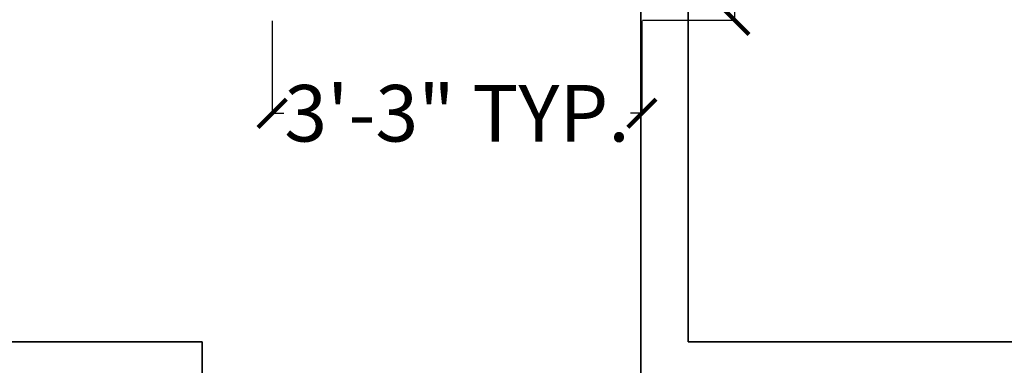
# Model space of a CAD drawing. Units: inches. Extents: x 844 to 2234, y 346 to 1084.
# Tile 66 of 93: x 1964 to 2069, y 632 to 669. Entities that reach past the tile are written whole.
import ezdxf

# ---------------------------------------------------------------- set-up
doc = ezdxf.new("R2010")
doc.units = ezdxf.units.IN
doc.header["$MEASUREMENT"] = 0
doc.layers.add('A-ANNO-DIMS', color=2, linetype='Continuous', lineweight=18)
doc.layers.add('A-WALL', color=7, linetype='Continuous', lineweight=35)
doc.styles.get("Standard").update_dxf_attribs({"font": 'arial.ttf'})
doc.dimstyles.get("Standard").update_dxf_attribs({"dimtxt": 6, "dimasz": 3, "dimexe": 0.18, "dimexo": 0.0625, "dimgap": 0.09, "dimtad": 0, "dimtih": 1, "dimtoh": 1, "dimdec": 1, "dimzin": 0, "dimdsep": 46, "dimlunit": 3, "dimtxsty": 'Standard', "dimblk": 'ARCHTICK', "dimcen": 0.09, "dimadec": 0, "dimazin": 0, "dimtfac": 1, "dimtdec": 1, "dimtofl": 0, "dimtmove": 0, "dimatfit": 3, "dimfxl": 1, "dimtolj": 1, "dimtzin": 0, "dimarcsym": 0})

# ---------------------------------------------------------------- blocks, each defined once
blk = doc.blocks.new('_ArchTick')
at = {"color": 0, "linetype": 'ByBlock', "const_width": 0.15}
blk.add_lwpolyline([(-0.5, -0.5), (0.5, 0.5)], dxfattribs=at)
blk = doc.blocks.new('*D121')
at = {"layer": 'A-ANNO-DIMS', "color": 0, "lineweight": -2, "transparency": 16777216}
for p, q in [((2030.27, 734.26), (2040.25, 734.26)), ((2040.07, 734.26), (2040.07, 704.6)), ((2040.07, 668.56), (2040.07, 698.22)), ((2030.27, 668.56), (2040.25, 668.56))]:
    blk.add_line(p, q, dxfattribs=at)
at = {"layer": 'Defpoints', "color": 0, "transparency": 16777216}
for p in [(2030.21, 734.26), (2040.07, 734.26), (2030.21, 668.56)]:
    blk.add_point(p, dxfattribs=at)
at = {"layer": 'A-ANNO-DIMS', "color": 0, "lineweight": -2, "transparency": 16777216, "xscale": 3, "yscale": 3, "zscale": 3}
for p, rotation in [((2040.07, 734.26), 90), ((2040.07, 668.56), 270)]:
    blk.add_blockref('_ArchTick', p, dxfattribs=dict(at, rotation=rotation))
at = {"layer": 'A-ANNO-DIMS', "color": 0, "transparency": 16777216, "insert": (2040.07, 701.41), "char_height": 6, "attachment_point": 5}
blk.add_mtext('\\A1;LOUNGE SET 5\'-5 1/2" TYP.', dxfattribs=at)
blk = doc.blocks.new('*D122')
at = {"layer": 'A-ANNO-DIMS', "color": 0, "lineweight": -2, "transparency": 16777216}
for p, q in [((1991.02, 668.49), (1991.02, 658.52)), ((2030.21, 668.49), (2030.21, 658.52)), ((1991.02, 658.7), (1992.24, 658.7)), ((2030.21, 658.7), (2028.99, 658.7))]:
    blk.add_line(p, q, dxfattribs=at)
at = {"layer": 'Defpoints', "color": 0, "transparency": 16777216}
for p in [(1991.02, 668.56), (2030.21, 668.56), (2030.21, 658.7)]:
    blk.add_point(p, dxfattribs=at)
at = {"layer": 'A-ANNO-DIMS', "color": 0, "lineweight": -2, "transparency": 16777216, "xscale": 3, "yscale": 3, "zscale": 3, "rotation": 180}
blk.add_blockref('_ArchTick', (1991.02, 658.7), dxfattribs=at)
at = {"layer": 'A-ANNO-DIMS', "color": 0, "lineweight": -2, "transparency": 16777216, "xscale": 3, "yscale": 3, "zscale": 3}
blk.add_blockref('_ArchTick', (2030.21, 658.7), dxfattribs=at)
at = {"layer": 'A-ANNO-DIMS', "color": 0, "transparency": 16777216, "insert": (2010.61, 658.7), "char_height": 6, "attachment_point": 5}
blk.add_mtext('\\A1;3\'-3" TYP.', dxfattribs=at)

msp = doc.modelspace()

# ---------------------------------------------------------------- linework, layer by layer
at = {"layer": 'A-WALL'}
for p, q in [((2030.1, 766.46), (2030.1, 629.46)), ((2035.1, 766.46), (2035.1, 634.46)), ((1939.1, 634.46), (1983.6, 634.46)), ((1983.6, 634.46), (1983.6, 521.46)), ((2167.1, 634.46), (2035.1, 634.46))]:
    msp.add_line(p, q, dxfattribs=at)

# ---------------------------------------------------------------- dimensions: what is measured, and where the dimension line sits
at = {"layer": 'A-ANNO-DIMS'}
dim = msp.add_linear_dim(base=(2040.07, 734.26), p1=(2030.21, 668.56), p2=(2030.21, 734.26), angle=90, text='LOUNGE SET <> TYP.', dimstyle='Standard', override={"dimdec": 1, "dimlfac": 1, "dimrnd": 0, "dimzin": 1, "dimdsep": 46, "dimlunit": 4, "dimfrac": 2}, dxfattribs=at)
dim.commit()
dim.dimension.update_dxf_attribs({"geometry": '*D121', "text_midpoint": (2040.07, 701.41)})
dim = msp.add_linear_dim(base=(2030.21, 658.7), p1=(1991.02, 668.56), p2=(2030.21, 668.56), text='<> TYP.', dimstyle='Standard', override={"dimdec": 1, "dimlfac": 1, "dimrnd": 0, "dimzin": 1, "dimdsep": 46, "dimlunit": 4, "dimfrac": 2}, dxfattribs=at)
dim.commit()
dim.dimension.update_dxf_attribs({"geometry": '*D122', "text_midpoint": (2010.61, 658.7)})

doc.saveas('drawing.dxf')
